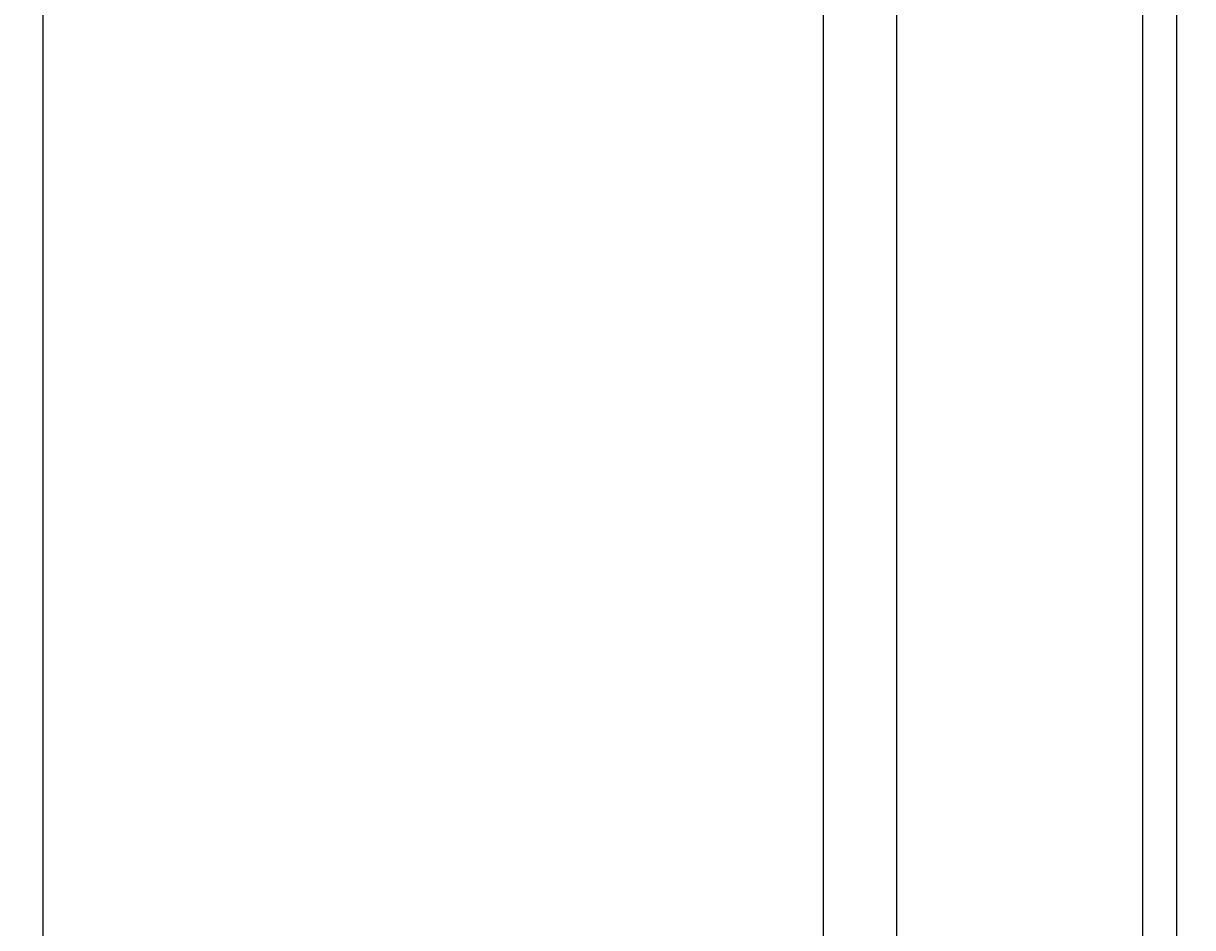
# Model space of a CAD drawing. Units: inches. Extents: x 35362 to 73946, y 43607 to 67532.
# Tile 124 of 134: x 50119 to 51337, y 49735 to 50677. Entities that reach past the tile are written whole.
import ezdxf

# ---------------------------------------------------------------- set-up
doc = ezdxf.new("R2010")
doc.units = ezdxf.units.IN
doc.header["$MEASUREMENT"] = 0
doc.layers.add('A-ANNO-DIMS', color=2, linetype='Continuous', lineweight=18)
doc.styles.get("Standard").update_dxf_attribs({"font": 'arial.ttf'})
doc.dimstyles.get("Standard").update_dxf_attribs({"dimtxt": 0.18, "dimasz": 0.18, "dimexe": 0.18, "dimexo": 0.0625, "dimgap": 0.09, "dimtad": 0, "dimtih": 1, "dimtoh": 1, "dimdec": 4, "dimzin": 0, "dimdsep": 46, "dimtxsty": 'Standard', "dimcen": 0.09, "dimadec": 0, "dimazin": 0, "dimtfac": 1, "dimtdec": 4, "dimtofl": 0, "dimtmove": 0, "dimatfit": 3, "dimfxl": 1, "dimtolj": 1, "dimtzin": 0, "dimarcsym": 0})

# ---------------------------------------------------------------- blocks, each defined once
blk = doc.blocks.new('*D11')
at = {"layer": 'A-ANNO-DIMS', "color": 0, "lineweight": -2, "transparency": 16777216}
for p, q in [((47978.7, 56028.8), (47978.7, 43606.7)), ((53109.8, 56028.8), (53109.8, 43606.7)), ((47978.8, 43606.9), (50543.9, 43606.9)), ((53109.6, 43606.9), (50544.6, 43606.9))]:
    blk.add_line(p, q, dxfattribs=at)
at = {"layer": 'A-ANNO-DIMS', "color": 0, "transparency": 16777216}
for points in [[(47978.8, 43606.9), (47978.8, 43606.8), (47978.7, 43606.9)], [(53109.6, 43606.9), (53109.6, 43606.8), (53109.8, 43606.9)]]:
    blk.add_solid(points, dxfattribs=at)
at = {"layer": 'Defpoints', "color": 0, "transparency": 16777216}
for p in [(47978.7, 56028.8), (53109.8, 56028.8), (53109.8, 43606.9)]:
    blk.add_point(p, dxfattribs=at)
at = {"layer": 'A-ANNO-DIMS', "color": 0, "transparency": 16777216, "insert": (50544.2, 43606.9), "char_height": 0.18, "attachment_point": 5}
blk.add_mtext('\\A1;5131', dxfattribs=at)
blk = doc.blocks.new('*D13')
at = {"layer": 'A-ANNO-DIMS', "color": 0, "lineweight": -2, "transparency": 16777216}
for p, q in [((48373.5, 51694), (48373.5, 43606.7)), ((51029, 51694), (51029, 43606.7)), ((48373.7, 43606.9), (49700.8, 43606.9)), ((51028.9, 43606.9), (49701.7, 43606.9))]:
    blk.add_line(p, q, dxfattribs=at)
at = {"layer": 'A-ANNO-DIMS', "color": 0, "transparency": 16777216}
for points in [[(48373.7, 43606.9), (48373.7, 43606.8), (48373.5, 43606.9)], [(51028.9, 43606.9), (51028.9, 43606.8), (51029, 43606.9)]]:
    blk.add_solid(points, dxfattribs=at)
at = {"layer": 'Defpoints', "color": 0, "transparency": 16777216}
for p in [(48373.5, 51694.1), (51029, 51694.1), (51029, 43606.9)]:
    blk.add_point(p, dxfattribs=at)
at = {"layer": 'A-ANNO-DIMS', "color": 0, "transparency": 16777216, "insert": (49701.3, 43606.9), "char_height": 0.18, "attachment_point": 5}
blk.add_mtext('\\A1;2655.6', dxfattribs=at)
blk = doc.blocks.new('*D17')
at = {"layer": 'A-ANNO-DIMS', "color": 0, "lineweight": -2, "transparency": 16777216}
for p, q in [((49923.3, 61293.2), (49923.3, 43606.7)), ((51913.9, 61293.2), (51913.9, 43606.7)), ((49923.5, 43606.9), (50918.2, 43606.9)), ((51913.8, 43606.9), (50919.1, 43606.9))]:
    blk.add_line(p, q, dxfattribs=at)
at = {"layer": 'A-ANNO-DIMS', "color": 0, "transparency": 16777216}
for points in [[(49923.5, 43606.9), (49923.5, 43606.8), (49923.3, 43606.9)], [(51913.8, 43606.9), (51913.8, 43606.8), (51913.9, 43606.9)]]:
    blk.add_solid(points, dxfattribs=at)
at = {"layer": 'Defpoints', "color": 0, "transparency": 16777216}
for p in [(49923.3, 61293.3), (51913.9, 61293.3), (51913.9, 43606.9)]:
    blk.add_point(p, dxfattribs=at)
at = {"layer": 'A-ANNO-DIMS', "color": 0, "transparency": 16777216, "insert": (50918.6, 43606.9), "char_height": 0.18, "attachment_point": 5}
blk.add_mtext('\\A1;1990.6', dxfattribs=at)
blk = doc.blocks.new('*D40')
at = {"layer": 'A-ANNO-DIMS', "color": 0, "lineweight": -2, "transparency": 16777216}
for p, q in [((56873.5, 53351.5), (35361.8, 53351.5)), ((35361.9, 53351.3), (35361.9, 51333.3)), ((35361.9, 49314.8), (35361.9, 51332.9)), ((51806.5, 49314.7), (35361.8, 49314.7))]:
    blk.add_line(p, q, dxfattribs=at)
at = {"layer": 'A-ANNO-DIMS', "color": 0, "transparency": 16777216}
for points in [[(35361.9, 53351.3), (35362, 53351.3), (35361.9, 53351.5)], [(35361.9, 49314.8), (35362, 49314.8), (35361.9, 49314.7)]]:
    blk.add_solid(points, dxfattribs=at)
at = {"layer": 'Defpoints', "color": 0, "transparency": 16777216}
for p in [(35361.9, 53351.5), (56873.6, 53351.5), (51806.5, 49314.7)]:
    blk.add_point(p, dxfattribs=at)
at = {"layer": 'A-ANNO-DIMS', "color": 0, "transparency": 16777216, "insert": (35361.9, 51333.1), "char_height": 0.18, "attachment_point": 5}
blk.add_mtext('\\A1;4036.9', dxfattribs=at)
blk = doc.blocks.new('*D67')
at = {"layer": 'A-ANNO-DIMS', "color": 0, "lineweight": -2, "transparency": 16777216}
for p, q in [((56873.5, 53351.5), (35361.8, 53351.5)), ((35361.9, 53351.3), (35361.9, 49400.9)), ((35361.9, 45450.1), (35361.9, 49400.5)), ((53793.6, 45449.9), (35361.8, 45449.9))]:
    blk.add_line(p, q, dxfattribs=at)
at = {"layer": 'A-ANNO-DIMS', "color": 0, "transparency": 16777216}
for points in [[(35361.9, 53351.3), (35362, 53351.3), (35361.9, 53351.5)], [(35361.9, 45450.1), (35362, 45450.1), (35361.9, 45449.9)]]:
    blk.add_solid(points, dxfattribs=at)
at = {"layer": 'Defpoints', "color": 0, "transparency": 16777216}
for p in [(35361.9, 53351.5), (56873.6, 53351.5), (53793.6, 45449.9)]:
    blk.add_point(p, dxfattribs=at)
at = {"layer": 'A-ANNO-DIMS', "color": 0, "transparency": 16777216, "insert": (35361.9, 49400.7), "char_height": 0.18, "attachment_point": 5}
blk.add_mtext('\\A1;7901.6', dxfattribs=at)
blk = doc.blocks.new('*D85')
at = {"layer": 'A-ANNO-DIMS', "color": 0, "lineweight": -2, "transparency": 16777216}
for p, q in [((50952.7, 49098.4), (50952.7, 67531.7)), ((50952.8, 67531.5), (51118.7, 67531.5)), ((51285.4, 67531.5), (51119.5, 67531.5)), ((51285.6, 49320.1), (51285.6, 67531.7))]:
    blk.add_line(p, q, dxfattribs=at)
at = {"layer": 'A-ANNO-DIMS', "color": 0, "transparency": 16777216}
for points in [[(50952.8, 67531.5), (50952.8, 67531.5), (50952.7, 67531.5)], [(51285.4, 67531.5), (51285.4, 67531.5), (51285.6, 67531.5)]]:
    blk.add_solid(points, dxfattribs=at)
at = {"layer": 'Defpoints', "color": 0, "transparency": 16777216}
for p in [(51285.6, 67531.5), (51285.6, 49320.1), (50952.7, 49098.4)]:
    blk.add_point(p, dxfattribs=at)
at = {"layer": 'A-ANNO-DIMS', "color": 0, "transparency": 16777216, "insert": (51119.1, 67531.5), "char_height": 0.18, "attachment_point": 5}
blk.add_mtext('\\A1;332.9', dxfattribs=at)
blk = doc.blocks.new('*D107')
at = {"layer": 'A-ANNO-DIMS', "color": 0, "lineweight": -2, "transparency": 16777216}
for p, q in [((50139.6, 59850), (50139.6, 43606.7)), ((51320.8, 59850), (51320.8, 43606.7)), ((50139.7, 43606.9), (50729.7, 43606.9)), ((51320.6, 43606.9), (50730.6, 43606.9))]:
    blk.add_line(p, q, dxfattribs=at)
at = {"layer": 'A-ANNO-DIMS', "color": 0, "transparency": 16777216}
for points in [[(50139.7, 43606.9), (50139.7, 43606.8), (50139.6, 43606.9)], [(51320.6, 43606.9), (51320.6, 43606.8), (51320.8, 43606.9)]]:
    blk.add_solid(points, dxfattribs=at)
at = {"layer": 'Defpoints', "color": 0, "transparency": 16777216}
for p in [(50139.6, 59850.1), (51320.8, 59850.1), (51320.8, 43606.9)]:
    blk.add_point(p, dxfattribs=at)
at = {"layer": 'A-ANNO-DIMS', "color": 0, "transparency": 16777216, "insert": (50730.2, 43606.9), "char_height": 0.18, "attachment_point": 5}
blk.add_mtext('\\A1;1181.3', dxfattribs=at)

msp = doc.modelspace()

# ---------------------------------------------------------------- dimensions: what is measured, and where the dimension line sits
at = {"layer": 'A-ANNO-DIMS'}
for base, p1, p2, override, picture, middle in [((51285.595, 67531.512), (50952.662, 49098.368), (51285.595, 49320.079), {"dimdec": 1, "dimlfac": 1, "dimrnd": 0, "dimzin": 0, "dimdsep": 46, "dimlunit": 2}, '*D85', (51119.128, 67531.512)), ((51913.931, 43606.859), (49923.307, 61293.286), (51913.931, 61293.286), {"dimdec": 1, "dimlfac": 1, "dimrnd": 0, "dimzin": 0, "dimdsep": 46, "dimlunit": 2}, '*D17', (50918.619, 43606.859)), ((51320.8133, 43606.859), (50139.5627, 59850.0769), (51320.8133, 59850.0769), {"dimdec": 1, "dimlfac": 1, "dimrnd": 0, "dimzin": 0, "dimdsep": 46, "dimlunit": 2}, '*D107', (50730.188, 43606.859)), ((53109.76, 43606.859), (47978.665, 56028.836), (53109.76, 56028.836), {"dimdec": 0, "dimlfac": 1, "dimrnd": 0, "dimzin": 0, "dimdsep": 46, "dimlunit": 2}, '*D11', (50544.212, 43606.859)), ((51029.043, 43606.859), (48373.492, 51694.087), (51029.043, 51694.087), {"dimdec": 1, "dimlfac": 1, "dimrnd": 0, "dimzin": 0, "dimdsep": 46, "dimlunit": 2}, '*D13', (49701.267, 43606.859))]:
    dim = msp.add_linear_dim(base=base, p1=p1, p2=p2, dimstyle='Standard', override=override, dxfattribs=at)
    dim.commit()
    dim.dimension.update_dxf_attribs({"geometry": picture, "text_midpoint": middle})
for p1, picture, middle in [((51806.517, 49314.669), '*D40', (35361.949, 51333.099)), ((53793.638, 45449.894), '*D67', (35361.949, 49400.712))]:
    dim = msp.add_linear_dim(base=(35361.949, 53351.529), p1=p1, p2=(56873.602, 53351.529), angle=90, dimstyle='Standard', override={"dimdec": 1, "dimlfac": 1, "dimrnd": 0, "dimzin": 0, "dimdsep": 46, "dimlunit": 2}, dxfattribs=at)
    dim.commit()
    dim.dimension.update_dxf_attribs({"geometry": picture, "text_midpoint": middle})

doc.saveas('drawing.dxf')
